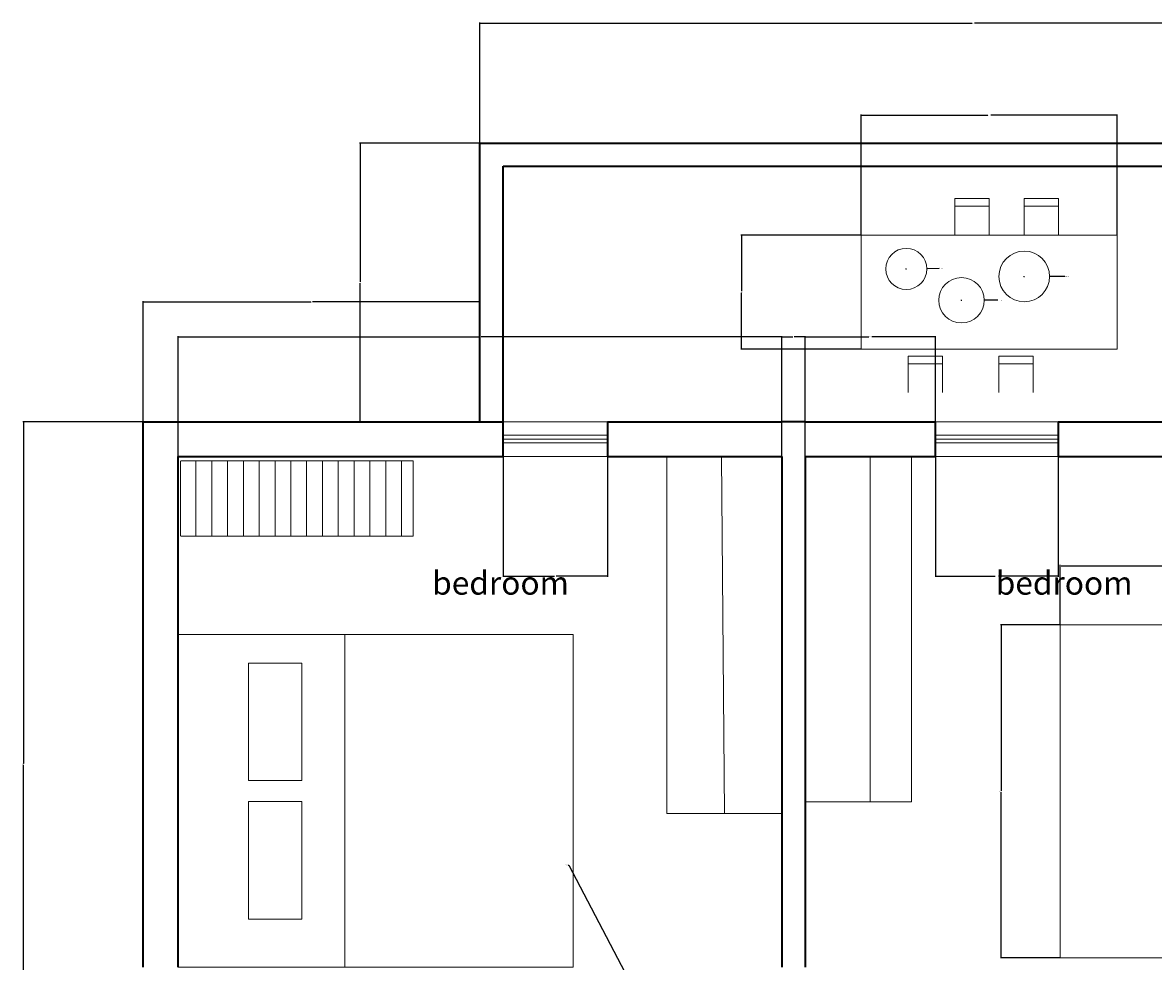
# Model space of a CAD drawing. Units: inches. Extents: x 177 to 785, y -381 to 206.
# Tile 3 of 5: x 237 to 529, y -37 to 206. Entities that reach past the tile are written whole.
import ezdxf

# ---------------------------------------------------------------- set-up
doc = ezdxf.new("R2010")
doc.units = ezdxf.units.IN
doc.header["$MEASUREMENT"] = 0
for name, color, linetype, lineweight in [('A-ANNO-DIMS', 2, 'Continuous', 18), ('A-AREA-IDEN', 7, 'Continuous', 20), ('A-FLOR-CASE', 9, 'Continuous', 20), ('A-FLOR-CASE-PATT', 9, 'Continuous', 13), ('A-FURN', 2, 'Continuous', 18), ('A-GLAZ', 4, 'Continuous', 18), ('A-WALL', 7, 'Continuous', 35)]:
    doc.layers.add(name, color=color, linetype=linetype, lineweight=lineweight)
doc.styles.get("Standard").update_dxf_attribs({"font": 'arial.ttf'})
doc.dimstyles.get("Standard").update_dxf_attribs({"dimtxt": 0.18, "dimasz": 0.18, "dimexe": 0.18, "dimexo": 0.0625, "dimgap": 0.09, "dimtad": 0, "dimtih": 1, "dimtoh": 1, "dimdec": 4, "dimzin": 0, "dimdsep": 46, "dimtxsty": 'Standard', "dimcen": 0.09, "dimadec": 0, "dimazin": 0, "dimtfac": 1, "dimtdec": 4, "dimtofl": 0, "dimtmove": 0, "dimatfit": 3, "dimfxl": 1, "dimtolj": 1, "dimtzin": 0, "dimarcsym": 0})

# ---------------------------------------------------------------- blocks, each defined once
blk = doc.blocks.new('BED-DOUBLE')
blk.add_line((58.96, 86.04), (58.96, 0))
for points in [[(0, 86.04), (102.05, 86.04), (102.05, 0), (0, 0)], [(70.1, 73.56), (83.84, 73.56), (83.84, 43.2), (70.1, 43.2)], [(70.1, 37.79), (83.84, 37.79), (83.84, 7.42), (70.1, 7.42)]]:
    blk.add_lwpolyline(points, close=True)
blk = doc.blocks.new('CHAIR-DINING')
for p, q in [((0, 9.42), (8.88, 9.42)), ((0, 7.42), (0, 9.42)), ((8.88, 9.42), (8.88, 7.42)), ((0, 0), (0, 7.42)), ((0, 7.42), (8.88, 7.42)), ((8.88, 7.42), (8.88, 0))]:
    blk.add_line(p, q)
blk = doc.blocks.new('*D13')
at = {"layer": 'A-ANNO-DIMS', "color": 0, "lineweight": -2, "transparency": 16777216}
for p, q in [((505.28, 50.4), (505.28, 65.83)), ((505.46, 65.65), (554.86, 65.65)), ((607.15, 65.65), (557.74, 65.65)), ((607.33, 50.4), (607.33, 65.83))]:
    blk.add_line(p, q, dxfattribs=at)
at = {"layer": 'A-ANNO-DIMS', "color": 0, "transparency": 16777216}
for points in [[(505.46, 65.68), (505.46, 65.62), (505.28, 65.65)], [(607.15, 65.68), (607.15, 65.62), (607.33, 65.65)]]:
    blk.add_solid(points, dxfattribs=at)
at = {"layer": 'Defpoints', "color": 0, "transparency": 16777216}
for p in [(607.33, 65.65), (505.28, 50.34), (607.33, 50.34)]:
    blk.add_point(p, dxfattribs=at)
at = {"layer": 'A-ANNO-DIMS', "color": 0, "transparency": 16777216, "insert": (556.3, 65.65), "char_height": 0.18, "attachment_point": 5}
blk.add_mtext('\\A1;DOUBLE BED 102 TYP.', dxfattribs=at)
blk = doc.blocks.new('*D14')
at = {"layer": 'A-ANNO-DIMS', "color": 0, "lineweight": -2, "transparency": 16777216}
for p, q in [((505.21, 50.34), (489.79, 50.34)), ((489.97, 50.16), (489.97, 7.5)), ((489.97, -35.53), (489.97, 7.13)), ((505.21, -35.71), (489.79, -35.71))]:
    blk.add_line(p, q, dxfattribs=at)
at = {"layer": 'A-ANNO-DIMS', "color": 0, "transparency": 16777216}
for points in [[(489.94, 50.16), (490, 50.16), (489.97, 50.34)], [(489.94, -35.53), (490, -35.53), (489.97, -35.71)]]:
    blk.add_solid(points, dxfattribs=at)
at = {"layer": 'Defpoints', "color": 0, "transparency": 16777216}
for p in [(489.97, 50.34), (505.28, 50.34), (505.28, -35.71)]:
    blk.add_point(p, dxfattribs=at)
at = {"layer": 'A-ANNO-DIMS', "color": 0, "transparency": 16777216, "insert": (489.97, 7.32), "char_height": 0.18, "attachment_point": 5}
blk.add_mtext('\\A1;86 TYP.', dxfattribs=at)
blk = doc.blocks.new('*D26')
at = {"layer": 'A-ANNO-DIMS', "color": 0, "lineweight": -2, "transparency": 16777216}
for p, q in [((268.33, 102.92), (268.33, 133.99)), ((268.51, 133.81), (311.61, 133.81)), ((355.15, 133.81), (312.05, 133.81)), ((355.33, 102.92), (355.33, 133.99))]:
    blk.add_line(p, q, dxfattribs=at)
at = {"layer": 'A-ANNO-DIMS', "color": 0, "transparency": 16777216}
for points in [[(268.51, 133.84), (268.51, 133.78), (268.33, 133.81)], [(355.15, 133.84), (355.15, 133.78), (355.33, 133.81)]]:
    blk.add_solid(points, dxfattribs=at)
at = {"layer": 'Defpoints', "color": 0, "transparency": 16777216}
for p in [(355.33, 133.81), (268.33, 102.86), (355.33, 102.86)]:
    blk.add_point(p, dxfattribs=at)
at = {"layer": 'A-ANNO-DIMS', "color": 0, "transparency": 16777216, "insert": (311.83, 133.81), "char_height": 0.18, "attachment_point": 5}
blk.add_mtext('\\A1;87', dxfattribs=at)
blk = doc.blocks.new('*D27')
at = {"layer": 'A-ANNO-DIMS', "color": 0, "lineweight": -2, "transparency": 16777216}
for p, q in [((355.33, 174.92), (355.33, 205.99)), ((355.51, 205.81), (482.54, 205.81)), ((610.15, 205.81), (483.12, 205.81)), ((610.33, 174.92), (610.33, 205.99))]:
    blk.add_line(p, q, dxfattribs=at)
at = {"layer": 'A-ANNO-DIMS', "color": 0, "transparency": 16777216}
for points in [[(355.51, 205.84), (355.51, 205.78), (355.33, 205.81)], [(610.15, 205.84), (610.15, 205.78), (610.33, 205.81)]]:
    blk.add_solid(points, dxfattribs=at)
at = {"layer": 'Defpoints', "color": 0, "transparency": 16777216}
for p in [(610.33, 205.81), (355.33, 174.86), (610.33, 174.86)]:
    blk.add_point(p, dxfattribs=at)
at = {"layer": 'A-ANNO-DIMS', "color": 0, "transparency": 16777216, "insert": (482.83, 205.81), "char_height": 0.18, "attachment_point": 5}
blk.add_mtext('\\A1;255', dxfattribs=at)
blk = doc.blocks.new('*D31')
at = {"layer": 'A-ANNO-DIMS', "color": 0, "lineweight": -2, "transparency": 16777216}
for p, q in [((355.27, 174.86), (324.2, 174.86)), ((324.38, 174.68), (324.38, 139.04)), ((324.38, 103.04), (324.38, 138.68)), ((355.27, 102.86), (324.2, 102.86))]:
    blk.add_line(p, q, dxfattribs=at)
at = {"layer": 'A-ANNO-DIMS', "color": 0, "transparency": 16777216}
for points in [[(324.35, 174.68), (324.41, 174.68), (324.38, 174.86)], [(324.35, 103.04), (324.41, 103.04), (324.38, 102.86)]]:
    blk.add_solid(points, dxfattribs=at)
at = {"layer": 'Defpoints', "color": 0, "transparency": 16777216}
for p in [(324.38, 174.86), (355.33, 174.86), (355.33, 102.86)]:
    blk.add_point(p, dxfattribs=at)
at = {"layer": 'A-ANNO-DIMS', "color": 0, "transparency": 16777216, "insert": (324.38, 138.86), "char_height": 0.18, "attachment_point": 5}
blk.add_mtext('\\A1;72', dxfattribs=at)
blk = doc.blocks.new('*D32')
at = {"layer": 'A-ANNO-DIMS', "color": 0, "lineweight": -2, "transparency": 16777216}
for p, q in [((277.33, 93.92), (277.33, 124.99)), ((277.51, 124.81), (355.05, 124.81)), ((433.15, 124.81), (355.61, 124.81)), ((433.33, 93.92), (433.33, 124.99))]:
    blk.add_line(p, q, dxfattribs=at)
at = {"layer": 'A-ANNO-DIMS', "color": 0, "transparency": 16777216}
for points in [[(277.51, 124.84), (277.51, 124.78), (277.33, 124.81)], [(433.15, 124.84), (433.15, 124.78), (433.33, 124.81)]]:
    blk.add_solid(points, dxfattribs=at)
at = {"layer": 'Defpoints', "color": 0, "transparency": 16777216}
for p in [(433.33, 124.81), (277.33, 93.86), (433.33, 93.86)]:
    blk.add_point(p, dxfattribs=at)
at = {"layer": 'A-ANNO-DIMS', "color": 0, "transparency": 16777216, "insert": (355.33, 124.81), "char_height": 0.18, "attachment_point": 5}
blk.add_mtext('\\A1;156', dxfattribs=at)
blk = doc.blocks.new('*D34')
at = {"layer": 'A-ANNO-DIMS', "color": 0, "lineweight": -2, "transparency": 16777216}
for p, q in [((361.33, 93.8), (361.33, 62.73)), ((388.33, 93.8), (388.33, 62.73)), ((361.51, 62.91), (374.61, 62.91)), ((388.15, 62.91), (375.05, 62.91))]:
    blk.add_line(p, q, dxfattribs=at)
at = {"layer": 'A-ANNO-DIMS', "color": 0, "transparency": 16777216}
for points in [[(361.51, 62.94), (361.51, 62.88), (361.33, 62.91)], [(388.15, 62.94), (388.15, 62.88), (388.33, 62.91)]]:
    blk.add_solid(points, dxfattribs=at)
at = {"layer": 'Defpoints', "color": 0, "transparency": 16777216}
for p in [(361.33, 93.86), (388.33, 93.86), (361.33, 62.91)]:
    blk.add_point(p, dxfattribs=at)
at = {"layer": 'A-ANNO-DIMS', "color": 0, "transparency": 16777216, "insert": (374.83, 62.91), "char_height": 0.18, "attachment_point": 5}
blk.add_mtext('\\A1;27', dxfattribs=at)
blk = doc.blocks.new('*D35')
at = {"layer": 'A-ANNO-DIMS', "color": 0, "lineweight": -2, "transparency": 16777216}
for p, q in [((473.05, 93.8), (473.05, 62.73)), ((504.71, 93.8), (504.71, 62.73)), ((473.23, 62.91), (488.48, 62.91)), ((504.53, 62.91), (489.27, 62.91))]:
    blk.add_line(p, q, dxfattribs=at)
at = {"layer": 'A-ANNO-DIMS', "color": 0, "transparency": 16777216}
for points in [[(473.23, 62.94), (473.23, 62.88), (473.05, 62.91)], [(504.53, 62.94), (504.53, 62.88), (504.71, 62.91)]]:
    blk.add_solid(points, dxfattribs=at)
at = {"layer": 'Defpoints', "color": 0, "transparency": 16777216}
for p in [(473.05, 93.86), (504.71, 93.86), (473.05, 62.91)]:
    blk.add_point(p, dxfattribs=at)
at = {"layer": 'A-ANNO-DIMS', "color": 0, "transparency": 16777216, "insert": (488.88, 62.91), "char_height": 0.18, "attachment_point": 5}
blk.add_mtext('\\A1;31.66', dxfattribs=at)
blk = doc.blocks.new('*D36')
at = {"layer": 'A-ANNO-DIMS', "color": 0, "lineweight": -2, "transparency": 16777216}
for p, q in [((439.33, 93.92), (439.33, 124.99)), ((439.51, 124.81), (455.8, 124.81)), ((472.87, 124.81), (456.58, 124.81)), ((473.05, 93.92), (473.05, 124.99))]:
    blk.add_line(p, q, dxfattribs=at)
at = {"layer": 'A-ANNO-DIMS', "color": 0, "transparency": 16777216}
for points in [[(439.51, 124.84), (439.51, 124.78), (439.33, 124.81)], [(472.87, 124.84), (472.87, 124.78), (473.05, 124.81)]]:
    blk.add_solid(points, dxfattribs=at)
at = {"layer": 'Defpoints', "color": 0, "transparency": 16777216}
for p in [(473.05, 124.81), (439.33, 93.86), (473.05, 93.86)]:
    blk.add_point(p, dxfattribs=at)
at = {"layer": 'A-ANNO-DIMS', "color": 0, "transparency": 16777216, "insert": (456.19, 124.81), "char_height": 0.18, "attachment_point": 5}
blk.add_mtext('\\A1;33.72', dxfattribs=at)
blk = doc.blocks.new('*D37')
at = {"layer": 'A-ANNO-DIMS', "color": 0, "lineweight": -2, "transparency": 16777216}
for p, q in [((268.27, 102.86), (237.2, 102.86)), ((237.38, 102.68), (237.38, 14.54)), ((237.38, -73.96), (237.38, 14.18)), ((268.27, -74.14), (237.2, -74.14))]:
    blk.add_line(p, q, dxfattribs=at)
at = {"layer": 'A-ANNO-DIMS', "color": 0, "transparency": 16777216}
for points in [[(237.35, 102.68), (237.41, 102.68), (237.38, 102.86)], [(237.35, -73.96), (237.41, -73.96), (237.38, -74.14)]]:
    blk.add_solid(points, dxfattribs=at)
at = {"layer": 'Defpoints', "color": 0, "transparency": 16777216}
for p in [(237.38, 102.86), (268.33, 102.86), (268.33, -74.14)]:
    blk.add_point(p, dxfattribs=at)
at = {"layer": 'A-ANNO-DIMS', "color": 0, "transparency": 16777216, "insert": (237.38, 14.36), "char_height": 0.18, "attachment_point": 5}
blk.add_mtext('\\A1;177', dxfattribs=at)
blk = doc.blocks.new('*D64')
at = {"layer": 'A-ANNO-DIMS', "color": 0, "lineweight": -2, "transparency": 16777216}
for p, q in [((433.33, 93.92), (433.33, 124.99)), ((433.51, 124.81), (436.18, 124.81)), ((439.15, 124.81), (436.48, 124.81)), ((439.33, 93.92), (439.33, 124.99))]:
    blk.add_line(p, q, dxfattribs=at)
at = {"layer": 'A-ANNO-DIMS', "color": 0, "transparency": 16777216}
for points in [[(433.51, 124.84), (433.51, 124.78), (433.33, 124.81)], [(439.15, 124.84), (439.15, 124.78), (439.33, 124.81)]]:
    blk.add_solid(points, dxfattribs=at)
at = {"layer": 'Defpoints', "color": 0, "transparency": 16777216}
for p in [(439.33, 124.81), (433.33, 93.86), (439.33, 93.86)]:
    blk.add_point(p, dxfattribs=at)
at = {"layer": 'A-ANNO-DIMS', "color": 0, "transparency": 16777216, "insert": (436.33, 124.81), "char_height": 0.18, "attachment_point": 5}
blk.add_mtext('\\A1;6', dxfattribs=at)
blk = doc.blocks.new('*D71')
at = {"layer": 'A-ANNO-DIMS', "color": 0, "lineweight": -2, "transparency": 16777216}
for p, q in [((453.86, 151.16), (453.86, 182.23)), ((454.04, 182.05), (486.53, 182.05)), ((519.81, 182.05), (487.32, 182.05)), ((519.99, 151.16), (519.99, 182.23))]:
    blk.add_line(p, q, dxfattribs=at)
at = {"layer": 'A-ANNO-DIMS', "color": 0, "transparency": 16777216}
for points in [[(454.04, 182.08), (454.04, 182.02), (453.86, 182.05)], [(519.81, 182.08), (519.81, 182.02), (519.99, 182.05)]]:
    blk.add_solid(points, dxfattribs=at)
at = {"layer": 'Defpoints', "color": 0, "transparency": 16777216}
for p in [(519.99, 182.05), (453.86, 151.1), (519.99, 151.1)]:
    blk.add_point(p, dxfattribs=at)
at = {"layer": 'A-ANNO-DIMS', "color": 0, "transparency": 16777216, "insert": (486.93, 182.05), "char_height": 0.18, "attachment_point": 5}
blk.add_mtext('\\A1;66.13', dxfattribs=at)
blk = doc.blocks.new('*D72')
at = {"layer": 'A-ANNO-DIMS', "color": 0, "lineweight": -2, "transparency": 16777216}
for p, q in [((453.8, 151.1), (422.73, 151.1)), ((422.91, 150.92), (422.91, 136.55)), ((422.91, 121.81), (422.91, 136.18)), ((453.8, 121.63), (422.73, 121.63))]:
    blk.add_line(p, q, dxfattribs=at)
at = {"layer": 'A-ANNO-DIMS', "color": 0, "transparency": 16777216}
for points in [[(422.88, 150.92), (422.94, 150.92), (422.91, 151.1)], [(422.88, 121.81), (422.94, 121.81), (422.91, 121.63)]]:
    blk.add_solid(points, dxfattribs=at)
at = {"layer": 'Defpoints', "color": 0, "transparency": 16777216}
for p in [(422.91, 151.1), (453.86, 151.1), (453.86, 121.63)]:
    blk.add_point(p, dxfattribs=at)
at = {"layer": 'A-ANNO-DIMS', "color": 0, "transparency": 16777216, "insert": (422.91, 136.37), "char_height": 0.18, "attachment_point": 5}
blk.add_mtext('\\A1;29.466', dxfattribs=at)
blk = doc.blocks.new('*D74')
at = {"layer": 'A-ANNO-DIMS', "color": 0, "lineweight": -2, "transparency": 16777216}
for p, q in [((378.1, -11.7), (378.28, -11.7)), ((378.28, -11.7), (395.76, -45.08)), ((425.02, -101.14), (425.2, -101.14)), ((425.11, -101.23), (425.11, -101.05))]:
    blk.add_line(p, q, dxfattribs=at)
at = {"layer": 'A-ANNO-DIMS', "color": 0, "transparency": 16777216}
blk.add_solid([(395.78, -45.07), (395.73, -45.1), (395.84, -45.24)], dxfattribs=at)
at = {"layer": 'Defpoints', "color": 0, "transparency": 16777216}
for p in [(395.84, -45.24), (425.11, -101.14)]:
    blk.add_point(p, dxfattribs=at)
at = {"layer": 'A-ANNO-DIMS', "color": 0, "transparency": 16777216, "insert": (377.7, -11.7), "char_height": 0.18, "attachment_point": 5}
blk.add_mtext('\\A1;R63.1', dxfattribs=at)
blk = doc.blocks.new('*D83')
at = {"layer": 'A-ANNO-DIMS', "color": 0, "lineweight": -2, "transparency": 16777216}
for p, q in [((495.88, 140.38), (496.06, 140.38)), ((495.97, 140.29), (495.97, 140.47)), ((506.45, 140.38), (502.7, 140.38))]:
    blk.add_line(p, q, dxfattribs=at)
at = {"layer": 'A-ANNO-DIMS', "color": 0, "transparency": 16777216}
blk.add_solid([(502.7, 140.41), (502.7, 140.35), (502.52, 140.38)], dxfattribs=at)
at = {"layer": 'Defpoints', "color": 0, "transparency": 16777216}
for p in [(489.42, 140.38), (502.52, 140.38)]:
    blk.add_point(p, dxfattribs=at)
at = {"layer": 'A-ANNO-DIMS', "color": 0, "transparency": 16777216, "insert": (507.01, 140.38), "char_height": 0.18, "attachment_point": 5}
blk.add_mtext('\\A1;∅13.097', dxfattribs=at)
blk = doc.blocks.new('*D84')
at = {"layer": 'A-ANNO-DIMS', "color": 0, "lineweight": -2, "transparency": 16777216}
for p, q in [((479.66, 134.24), (479.84, 134.24)), ((479.75, 134.15), (479.75, 134.33)), ((489.15, 134.24), (485.81, 134.24))]:
    blk.add_line(p, q, dxfattribs=at)
at = {"layer": 'A-ANNO-DIMS', "color": 0, "transparency": 16777216}
blk.add_solid([(485.81, 134.27), (485.81, 134.21), (485.63, 134.24)], dxfattribs=at)
at = {"layer": 'Defpoints', "color": 0, "transparency": 16777216}
for p in [(473.88, 134.24), (485.63, 134.24)]:
    blk.add_point(p, dxfattribs=at)
at = {"layer": 'A-ANNO-DIMS', "color": 0, "transparency": 16777216, "insert": (489.71, 134.24), "char_height": 0.18, "attachment_point": 5}
blk.add_mtext('\\A1;∅11.743', dxfattribs=at)
blk = doc.blocks.new('*D85')
at = {"layer": 'A-ANNO-DIMS', "color": 0, "lineweight": -2, "transparency": 16777216}
for p, q in [((465.4, 142.34), (465.58, 142.34)), ((465.49, 142.25), (465.49, 142.43)), ((473.99, 142.43), (470.98, 142.4))]:
    blk.add_line(p, q, dxfattribs=at)
at = {"layer": 'A-ANNO-DIMS', "color": 0, "transparency": 16777216}
blk.add_solid([(470.98, 142.43), (470.98, 142.37), (470.8, 142.4)], dxfattribs=at)
at = {"layer": 'Defpoints', "color": 0, "transparency": 16777216}
for p in [(460.19, 142.28), (470.8, 142.4)]:
    blk.add_point(p, dxfattribs=at)
at = {"layer": 'A-ANNO-DIMS', "color": 0, "transparency": 16777216, "insert": (474.55, 142.43), "char_height": 0.18, "attachment_point": 5}
blk.add_mtext('\\A1;∅10.617', dxfattribs=at)

msp = doc.modelspace()

# ---------------------------------------------------------------- hatches: boundary and pattern name
at = {"layer": 'A-FLOR-CASE-PATT'}
h = msp.add_hatch(dxfattribs=at)
h.set_pattern_fill('ANSI31', color=256, scale=32.69, angle=45, style=0)
h.paths.add_polyline_path([(278.1025, 73.2758), (338.1025, 73.2758), (338.1025, 92.7046), (278.1025, 92.7046)])

# ---------------------------------------------------------------- linework, layer by layer
at = {"layer": 'A-FLOR-CASE'}
for p, q in [((403.6328, 93.8599), (403.6328, 1.6186)), ((417.7209, 93.8599), (418.4806, 1.6186)), ((456.188, 93.8599), (456.188, 4.6048)), ((466.8155, 93.8599), (466.8155, 4.6048)), ((277.9563, 73.2758), (277.9563, 92.7046)), ((338.1025, 92.7046), (278.1025, 92.7046)), ((338.1025, 92.7046), (338.1025, 73.2758)), ((338.1025, 73.2758), (278.1025, 73.2758)), ((466.8155, 4.6048), (439.3284, 4.6048)), ((403.6328, 1.6186), (433.3284, 1.6186))]:
    msp.add_line(p, q, dxfattribs=at)
at = {"layer": 'A-FURN'}
msp.add_lwpolyline([(453.8639, 151.099), (519.9891, 151.099), (519.9891, 121.6325), (453.8639, 121.6325)], close=True, dxfattribs=at)
for centre, radius in [((465.4945, 142.339), 5.3084), ((495.9707, 140.3833), 6.5483), ((479.754, 134.2367), 5.8716)]:
    msp.add_circle(centre, radius, dxfattribs=at)
at = {"layer": 'A-GLAZ'}
for p, q in [((388.3284, 99.3599), (361.3284, 99.3599)), ((504.7052, 99.3599), (473.0475, 99.3599)), ((388.3284, 98.3599), (361.3284, 98.3599)), ((388.3284, 97.3599), (361.3284, 97.3599)), ((504.7052, 98.3599), (473.0475, 98.3599)), ((504.7052, 97.3599), (473.0475, 97.3599))]:
    msp.add_line(p, q, dxfattribs=at)
for points in [[(361.3284, 102.8599), (388.3284, 102.8599), (388.3284, 93.8599), (361.3284, 93.8599)], [(473.0475, 102.8599), (504.7052, 102.8599), (504.7052, 93.8599), (473.0475, 93.8599)]]:
    msp.add_lwpolyline(points, close=True, dxfattribs=at)
at = {"layer": 'A-WALL'}
for p, q in [((355.3284, 102.8599), (355.3284, 174.8599)), ((355.3284, 174.8599), (521.8284, 174.8599)), ((521.8284, 174.8599), (604.3284, 174.8599)), ((361.3284, 168.8599), (515.8284, 168.8599)), ((361.3284, 102.8599), (361.3284, 168.8599)), ((515.8284, 168.8599), (604.3284, 168.8599)), ((268.3284, 93.8599), (268.3284, 102.8599)), ((268.3284, 102.8599), (277.3284, 102.8599)), ((277.3284, 102.8599), (361.3284, 102.8599)), ((361.3284, 93.8599), (361.3284, 102.8599)), ((388.3284, 102.8599), (388.3284, 93.8599)), ((388.3284, 102.8599), (433.3284, 102.8599)), ((439.3284, 102.8599), (433.3284, 102.8599)), ((439.3284, 102.8599), (473.0475, 102.8599)), ((473.0475, 93.8599), (473.0475, 102.8599)), ((504.7052, 102.8599), (504.7052, 93.8599)), ((504.7052, 102.8599), (604.3284, 102.8599)), ((268.3284, -38.1401), (268.3284, 93.8599)), ((277.3284, -38.1401), (277.3284, 93.8599)), ((277.3284, 93.8599), (361.3284, 93.8599)), ((388.3284, 93.8599), (433.3284, 93.8599)), ((433.3284, 93.8599), (433.3284, -38.1401)), ((439.3284, 93.8599), (439.3284, -38.1401)), ((439.3284, 93.8599), (473.0475, 93.8599)), ((504.7052, 93.8599), (607.3284, 93.8599))]:
    msp.add_line(p, q, dxfattribs=at)

# ---------------------------------------------------------------- block references
at = {"layer": 'A-FURN'}
for name, p in [('CHAIR-DINING', (478.0468, 151.0991)), ('CHAIR-DINING', (495.9126, 151.0991)), ('CHAIR-DINING', (465.9899, 110.3723)), ('CHAIR-DINING', (489.4199, 110.3723)), ('BED-DOUBLE', (505.275, -35.706))]:
    msp.add_blockref(name, p, dxfattribs=at)
at = {"layer": 'A-FURN', "rotation": 180}
msp.add_blockref('BED-DOUBLE', (379.3818, 47.9038), dxfattribs=at)

# ---------------------------------------------------------------- texts
at = {"layer": 'A-AREA-IDEN', "char_height": 6, "attachment_point": 1}
for insert in [(342.9919, 64.165), (488.5921, 64.165)]:
    msp.add_mtext_dynamic_manual_height_columns('bedroom', width=20.406791, gutter_width=1, heights=[0], dxfattribs=dict(at, insert=insert))

# ---------------------------------------------------------------- dimensions: what is measured, and where the dimension line sits
at = {"layer": 'A-ANNO-DIMS'}
for base, p1, p2, override, picture, middle in [((610.3284, 205.8099), (355.3284, 174.8599), (610.3284, 174.8599), {"dimdec": 0, "dimlfac": 1, "dimrnd": 0, "dimzin": 0, "dimdsep": 46, "dimlunit": 2}, '*D27', (482.8284, 205.8099)), ((519.9891, 182.049), (453.8639, 151.099), (519.9891, 151.099), {"dimdec": 2, "dimlfac": 1, "dimrnd": 0, "dimzin": 0, "dimdsep": 46, "dimlunit": 2}, '*D71', (486.9265, 182.049)), ((355.3284, 133.8099), (268.3284, 102.8599), (355.3284, 102.8599), {"dimdec": 0, "dimlfac": 1, "dimrnd": 0, "dimzin": 0, "dimdsep": 46, "dimlunit": 2}, '*D26', (311.8284, 133.8099)), ((433.3284, 124.8099), (277.3284, 93.8599), (433.3284, 93.8599), {"dimdec": 0, "dimlfac": 1, "dimrnd": 0, "dimzin": 0, "dimdsep": 46, "dimlunit": 2}, '*D32', (355.3284, 124.8099)), ((439.3284, 124.8099), (433.3284, 93.8599), (439.3284, 93.8599), {"dimdec": 0, "dimlfac": 1, "dimrnd": 0, "dimzin": 0, "dimdsep": 46, "dimlunit": 2}, '*D64', (436.3284, 124.8099)), ((473.0475, 124.8099), (439.3284, 93.8599), (473.0475, 93.8599), {"dimdec": 2, "dimlfac": 1, "dimrnd": 0, "dimzin": 0, "dimdsep": 46, "dimlunit": 2}, '*D36', (456.188, 124.8099))]:
    dim = msp.add_linear_dim(base=base, p1=p1, p2=p2, dimstyle='Standard', override=override, dxfattribs=at)
    dim.commit()
    dim.dimension.update_dxf_attribs({"geometry": picture, "text_midpoint": middle})
for base, p1, p2, angle, override, picture, middle in [((324.3784, 174.8599), (355.3284, 102.8599), (355.3284, 174.8599), 90, {"dimdec": 0, "dimlfac": 1, "dimrnd": 0, "dimzin": 0, "dimdsep": 46, "dimlunit": 2}, '*D31', (324.3784, 138.8599)), ((422.91392, 151.09895), (453.86392, 121.63248), (453.86392, 151.09895), 90, {"dimdec": 3, "dimlfac": 1, "dimrnd": 0, "dimzin": 0, "dimdsep": 46, "dimlunit": 2}, '*D72', (422.91392, 136.36572)), ((237.3784, 102.8599), (268.3284, -74.1401), (268.3284, 102.8599), 90, {"dimdec": 0, "dimlfac": 1, "dimrnd": 0, "dimzin": 0, "dimdsep": 46, "dimlunit": 2}, '*D37', (237.3784, 14.3599)), ((361.3284, 62.9099), (388.3284, 93.8599), (361.3284, 93.8599), 180, {"dimdec": 0, "dimlfac": 1, "dimrnd": 0, "dimzin": 0, "dimdsep": 46, "dimlunit": 2}, '*D34', (374.8284, 62.9099)), ((473.0475, 62.9099), (504.7052, 93.8599), (473.0475, 93.8599), 180, {"dimdec": 2, "dimlfac": 1, "dimrnd": 0, "dimzin": 0, "dimdsep": 46, "dimlunit": 2}, '*D35', (488.8764, 62.9099))]:
    dim = msp.add_linear_dim(base=base, p1=p1, p2=p2, angle=angle, dimstyle='Standard', override=override, dxfattribs=at)
    dim.commit()
    dim.dimension.update_dxf_attribs({"geometry": picture, "text_midpoint": middle})
for p1, p2, picture, middle in [((460.1864, 142.2792), (470.8026, 142.3989), '*D85', (473.9874, 142.4348)), ((489.4223, 140.3836), (502.519, 140.383), '*D83', (506.448, 140.3828)), ((473.8824, 134.2364), (485.6255, 134.237), '*D84', (489.1485, 134.2372))]:
    dim = msp.add_diameter_dim_2p(p1=p1, p2=p2, dimstyle='Standard', override={"dimdec": 3, "dimlfac": 1, "dimrnd": 0, "dimzin": 0, "dimdsep": 46, "dimlunit": 2}, dxfattribs=at)
    dim.commit()
    dim.dimension.update_dxf_attribs({"geometry": picture, "text_midpoint": middle, "dimtype": 163})
dim = msp.add_linear_dim(base=(607.3284, 65.6459), p1=(505.2755, 50.3379), p2=(607.3284, 50.3379), text='DOUBLE BED <> TYP.', dimstyle='Standard', override={"dimdec": 0, "dimlfac": 1, "dimrnd": 0, "dimzin": 0, "dimdsep": 46, "dimlunit": 2}, dxfattribs=at)
dim.commit()
dim.dimension.update_dxf_attribs({"geometry": '*D13', "text_midpoint": (556.302, 65.6459)})
dim = msp.add_linear_dim(base=(489.9676, 50.3379), p1=(505.2755, -35.7056), p2=(505.2755, 50.3379), angle=90, text='<> TYP.', dimstyle='Standard', override={"dimdec": 0, "dimlfac": 1, "dimrnd": 0, "dimzin": 0, "dimdsep": 46, "dimlunit": 2}, dxfattribs=at)
dim.commit()
dim.dimension.update_dxf_attribs({"geometry": '*D14', "text_midpoint": (489.9676, 7.3162)})
dim = msp.add_radius_dim(center=(425.1088, -101.1401), mpoint=(395.839, -45.2419), dimstyle='Standard', override={"dimdec": 1, "dimlfac": 1, "dimrnd": 0, "dimzin": 0, "dimdsep": 46, "dimlunit": 2}, dxfattribs=at)
dim.commit()
dim.dimension.update_dxf_attribs({"geometry": '*D74', "text_midpoint": (377.7045, -11.703), "dimtype": 164})

doc.saveas('drawing.dxf')
